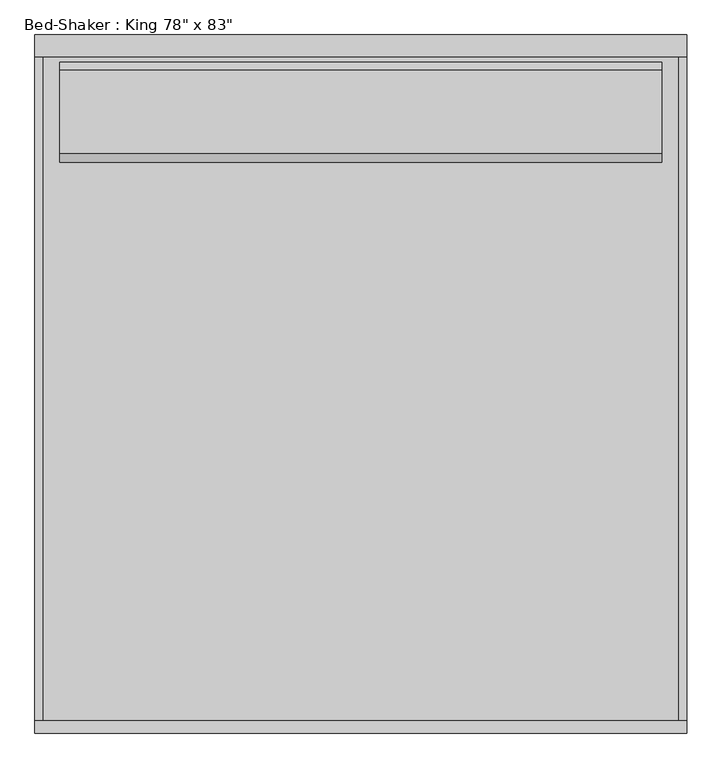
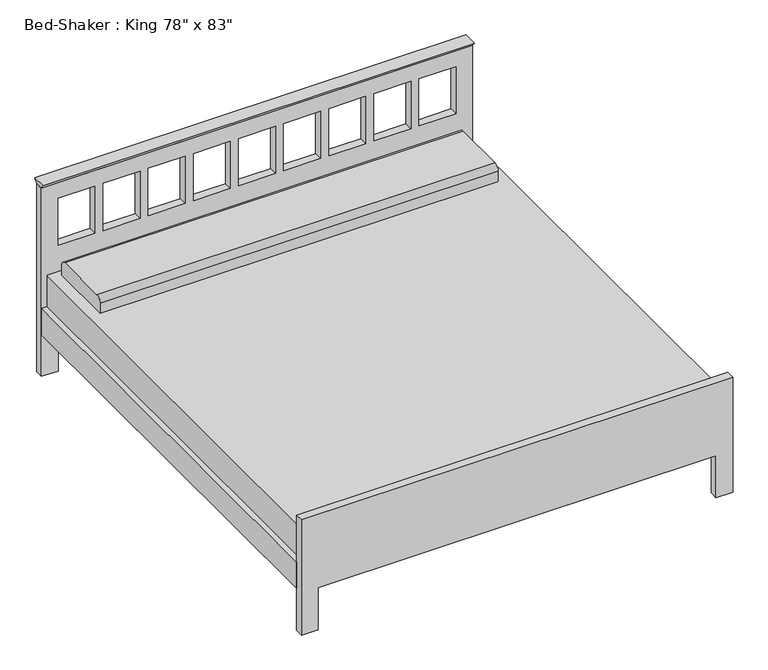
"""IFC4 building model written with IfcOpenShell, lengths in millimetres: furniture geometry."""

from ifc_helpers import new_model, si_unit, point, frame, frame_2d, origin, place, context, project, spatial, polyline, circle_curve, trimmed, segment, composite_curve, outline, extrude, source, transform, mapped, element, save


def furniture_29cd36cd(model_context):
    return source(origin(), model_context, "Body", "SweptSolid", [
        extrude(outline(polyline([(-38.1, 914.4), (-51.9545455, 933.45), (13.8545455, 933.45), (0.0, 914.4), (-38.1, 914.4)])), frame((-1009.4365546, 0.0, 0.0), z_axis=(1.0, 0.0, 0.0), x_axis=(0.0, 1.0, 0.0)), (0.0, 0.0, 1.0), 1981.2533613),
        extrude(outline(composite_curve([segment(polyline([(-373.2486637, 482.6), (-373.2486637, 533.4)]), True, "CONTINUOUS"), segment(trimmed(circle_curve(frame_2d((-347.8486637, 533.4)), 25.4), [point((-373.2486637, 533.4))], [point((-347.8486637, 558.8))], False, "CARTESIAN"), True, "CONTINUOUS"), segment(polyline([(-347.8486637, 558.8), (-93.8486637, 558.8)]), True, "CONTINUOUS"), segment(trimmed(circle_curve(frame_2d((-93.8486637, 533.4)), 25.4), [point((-93.8486637, 558.8))], [point((-68.4486637, 533.4))], False, "CARTESIAN"), True, "CONTINUOUS"), segment(polyline([(-68.4486637, 533.4), (-68.4486637, 482.6), (-373.2486637, 482.6)]), True, "CONTINUOUS")], self_intersect=False)), frame((-933.45, 0.0, 0.0), z_axis=(1.0, 0.0, 0.0), x_axis=(0.0, 1.0, 0.0)), (0.0, 0.0, 1.0), 1828.8),
        extrude(outline(polyline([(946.15, -38.1), (946.15, -2070.1), (-984.25, -2070.1), (-984.25, -38.1), (946.15, -38.1)])), frame((0.0, 0.0, 228.6), z_axis=(0.0, 0.0, 1.0), x_axis=(1.0, 0.0, 0.0)), (0.0, 0.0, 1.0), 254.0),
        extrude(outline(polyline([(946.15, -2070.1), (946.15, -38.1), (971.55, -38.1), (971.55, -2070.1), (946.15, -2070.1)])), frame((0.0, 0.0, 203.0994861), z_axis=(0.0, 0.0, 1.0), x_axis=(1.0, 0.0, 0.0)), (0.0, 0.0, 1.0), 127.0),
        extrude(outline(polyline([(-1009.65, -2070.1), (-1009.65, -38.1), (-984.25, -38.1), (-984.25, -2070.1), (-1009.65, -2070.1)])), frame((0.0, 0.0, 203.5755296), z_axis=(0.0, 0.0, 1.0), x_axis=(1.0, 0.0, 0.0)), (0.0, 0.0, 1.0), 127.0),
        extrude(outline(polyline([(0.0, -933.45), (203.2, -933.45), (203.2, 895.35), (0.0, 895.35), (0.0, 971.55), (558.8, 971.55), (558.8, -1009.65), (0.0, -1009.65), (0.0, -933.45)])), frame((0.0, -2108.2, 0.0), z_axis=(0.0, 1.0, 0.0), x_axis=(0.0, 0.0, 1.0)), (0.0, 0.0, 1.0), 38.1),
        extrude(outline(polyline([(914.4, 971.8168067), (914.4, -1009.4365546), (0.0, -1009.4365546), (0.0, -933.45), (203.2, -933.45), (203.2, 895.35), (0.0, 895.35), (0.0, 971.8168067), (914.4, 971.8168067)]), holes=[polyline([(838.2, -764.1166667), (609.6, -764.1166667), (609.6, -933.45), (838.2, -933.45), (838.2, -764.1166667)]), polyline([(838.2, -556.6833333), (609.6, -556.6833333), (609.6, -726.0166667), (838.2, -726.0166667), (838.2, -556.6833333)]), polyline([(838.2, -349.25), (609.6, -349.25), (609.6, -518.5833333), (838.2, -518.5833333), (838.2, -349.25)]), polyline([(838.2, -141.8166667), (609.6, -141.8166667), (609.6, -311.15), (838.2, -311.15), (838.2, -141.8166667)]), polyline([(838.2, 273.05), (609.6, 273.05), (609.6, 103.7166667), (838.2, 103.7166667), (838.2, 273.05)]), polyline([(838.2, 480.4833333), (609.6, 480.4833333), (609.6, 311.15), (838.2, 311.15), (838.2, 480.4833333)]), polyline([(838.2, 687.9166667), (609.6, 687.9166667), (609.6, 518.5833333), (838.2, 518.5833333), (838.2, 687.9166667)]), polyline([(838.2, 895.35), (609.6, 895.35), (609.6, 726.0166667), (838.2, 726.0166667), (838.2, 895.35)]), polyline([(838.2, 65.6166667), (609.6, 65.6166667), (609.6, -103.7166667), (838.2, -103.7166667), (838.2, 65.6166667)])]), frame((0.0, -38.1, 0.0), z_axis=(0.0, 1.0, 0.0), x_axis=(0.0, 0.0, 1.0)), (0.0, 0.0, 1.0), 38.1),
    ])


if __name__ == "__main__":
    model = new_model("IFC4")
    model_context = context("Model", 3, world=origin())
    ifc_project = project(units=[si_unit("LENGTHUNIT", "METRE", prefix="MILLI")], contexts=[model_context])
    site = spatial("IfcSite", under=ifc_project)
    building = spatial("IfcBuilding", under=site)
    placement = place(None, origin())
    furniture_shape = furniture_29cd36cd(model_context)
    element("IfcFurniture", 1, ObjectType="Bed-Shaker : King 78\" x 83\"", at=placement, inside=building, context=model_context, shape_type="MappedRepresentation", body=[
        mapped(furniture_shape, transform((0.0, 0.0, 0.0), x_axis=(1.0, 0.0, 0.0), y_axis=(0.0, 1.0, 0.0), z_axis=(0.0, 0.0, 1.0))),
    ])
    save(model, "model.ifc")

# Revit data of these elements
# Type "Bed-Shaker : King 78\" x 83\""
#   Assembly Code = "E2020200"
#   Length = 6' - 11"
#   Width = 6' - 6"
#   Frame Material = Birch
#   Mattress Material = Softwood, Lumber
#   Default Elevation = 0
# Element 1 (IfcFurniture, "Bed-Shaker : King 78\" x 83\"")
#   Materials on its faces: "Birch", "Softwood, Lumber"
# Materials
#   "Birch": class "Wood", colour RGB 224 178 126, transparency 0, Description = "Betula Alleghaniensis", Cost = 0
#   "Softwood, Lumber": class "Wood", colour RGB 223 192 134, transparency 0, Description = "Pinus Echinata", Cost = 0
